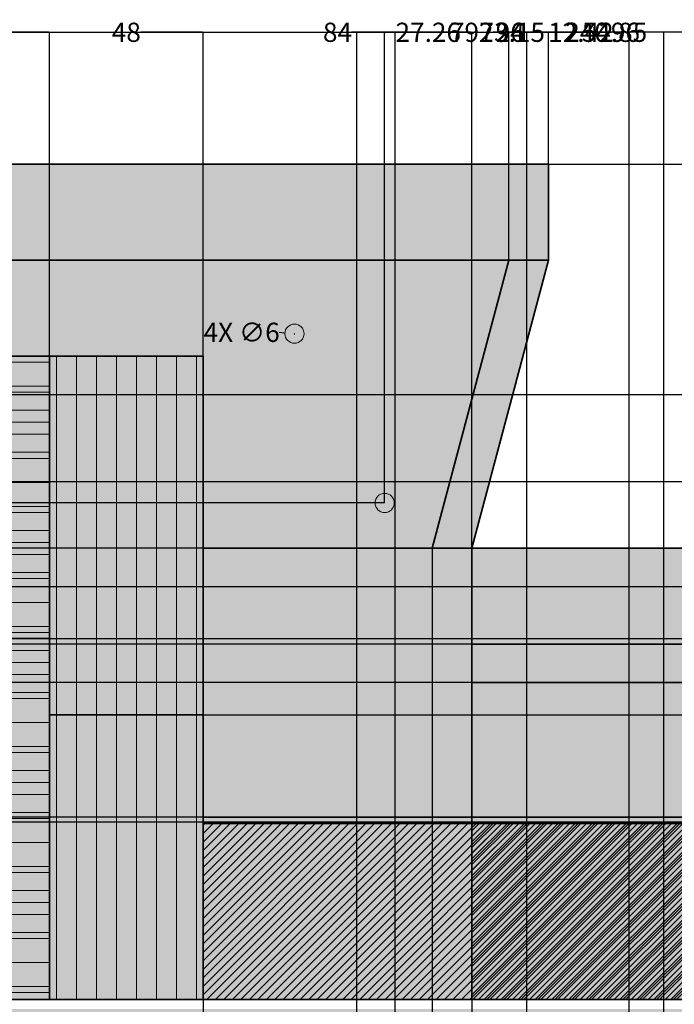
# Model space of a CAD drawing. Units: inches. Extents: x 148 to 1080, y 89 to 707.
# Tile 10 of 12: x 470 to 674, y 399 to 707. Entities that reach past the tile are written whole.
import ezdxf

# ---------------------------------------------------------------- set-up
doc = ezdxf.new("R2010")
doc.units = ezdxf.units.IN
doc.header["$MEASUREMENT"] = 0
for name, color, linetype, lineweight in [('A-ANNO-DIMS', 2, 'Continuous', 18), ('A-ELEV', 7, 'Continuous', 35), ('A-ELEV-PATT', 8, 'Continuous', 13), ('E-LITE', 3, 'Continuous', 18)]:
    doc.layers.add(name, color=color, linetype=linetype, lineweight=lineweight)
doc.styles.get("Standard").update_dxf_attribs({"font": 'arial.ttf'})
doc.dimstyles.get("Standard").update_dxf_attribs({"dimtxt": 6, "dimasz": 0.18, "dimexe": 0.18, "dimexo": 0.0625, "dimgap": 0.09, "dimtad": 0, "dimtih": 1, "dimtoh": 1, "dimdec": 0, "dimzin": 0, "dimdsep": 46, "dimlunit": 3, "dimtxsty": 'Standard', "dimcen": 0.09, "dimadec": 0, "dimazin": 0, "dimtfac": 1, "dimtdec": 0, "dimtofl": 0, "dimtmove": 0, "dimatfit": 3, "dimfxl": 1, "dimtolj": 1, "dimtzin": 0, "dimarcsym": 0})

# ---------------------------------------------------------------- blocks, each defined once
blk = doc.blocks.new('*D1')
at = {"layer": 'A-ANNO-DIMS', "color": 0, "lineweight": -2, "transparency": 16777216}
for p, q in [((215.02, 662.01), (215.02, 703.28)), ((215.2, 703.1), (604.32, 703.1)), ((1006.77, 703.1), (617.65, 703.1)), ((1006.95, 338.01), (1006.95, 703.28))]:
    blk.add_line(p, q, dxfattribs=at)
at = {"layer": 'A-ANNO-DIMS', "color": 0, "transparency": 16777216}
for points in [[(215.2, 703.13), (215.2, 703.07), (215.02, 703.1)], [(1006.77, 703.13), (1006.77, 703.07), (1006.95, 703.1)]]:
    blk.add_solid(points, dxfattribs=at)
at = {"layer": 'Defpoints', "color": 0, "transparency": 16777216}
for p in [(1006.95, 703.1), (215.02, 661.95), (1006.95, 337.95)]:
    blk.add_point(p, dxfattribs=at)
at = {"layer": 'A-ANNO-DIMS', "color": 0, "transparency": 16777216, "insert": (610.98, 703.1), "char_height": 6, "attachment_point": 5}
blk.add_mtext('\\A1;792', dxfattribs=at)
blk = doc.blocks.new('*D11')
at = {"layer": 'A-ANNO-DIMS', "color": 0, "lineweight": -2, "transparency": 16777216}
for p, q in [((395.02, 602.01), (395.02, 703.28)), ((395.2, 703.1), (432.64, 703.1)), ((478.84, 703.1), (441.4, 703.1)), ((479.02, 602.01), (479.02, 703.28))]:
    blk.add_line(p, q, dxfattribs=at)
at = {"layer": 'A-ANNO-DIMS', "color": 0, "transparency": 16777216}
for points in [[(395.2, 703.13), (395.2, 703.07), (395.02, 703.1)], [(478.84, 703.13), (478.84, 703.07), (479.02, 703.1)]]:
    blk.add_solid(points, dxfattribs=at)
at = {"layer": 'Defpoints', "color": 0, "transparency": 16777216}
for p in [(479.02, 703.1), (395.02, 601.95), (479.02, 601.95)]:
    blk.add_point(p, dxfattribs=at)
at = {"layer": 'A-ANNO-DIMS', "color": 0, "transparency": 16777216, "insert": (437.02, 703.1), "char_height": 6, "attachment_point": 5}
blk.add_mtext('\\A1;84', dxfattribs=at)
blk = doc.blocks.new('*D12')
at = {"layer": 'A-ANNO-DIMS', "color": 0, "lineweight": -2, "transparency": 16777216}
for p, q in [((479.02, 602.01), (479.02, 703.28)), ((479.2, 703.1), (498.51, 703.1)), ((526.84, 703.1), (507.53, 703.1)), ((527.02, 602.01), (527.02, 703.28))]:
    blk.add_line(p, q, dxfattribs=at)
at = {"layer": 'A-ANNO-DIMS', "color": 0, "transparency": 16777216}
for points in [[(479.2, 703.13), (479.2, 703.07), (479.02, 703.1)], [(526.84, 703.13), (526.84, 703.07), (527.02, 703.1)]]:
    blk.add_solid(points, dxfattribs=at)
at = {"layer": 'Defpoints', "color": 0, "transparency": 16777216}
for p in [(527.02, 703.1), (479.02, 601.95), (527.02, 601.95)]:
    blk.add_point(p, dxfattribs=at)
at = {"layer": 'A-ANNO-DIMS', "color": 0, "transparency": 16777216, "insert": (503.02, 703.1), "char_height": 6, "attachment_point": 5}
blk.add_mtext('\\A1;48', dxfattribs=at)
blk = doc.blocks.new('*D13')
at = {"layer": 'A-ANNO-DIMS', "color": 0, "lineweight": -2, "transparency": 16777216}
for p, q in [((527.02, 542.01), (527.02, 703.28)), ((527.2, 703.1), (564.64, 703.1)), ((610.84, 703.1), (573.4, 703.1)), ((611.02, 542.01), (611.02, 703.28))]:
    blk.add_line(p, q, dxfattribs=at)
at = {"layer": 'A-ANNO-DIMS', "color": 0, "transparency": 16777216}
for points in [[(527.2, 703.13), (527.2, 703.07), (527.02, 703.1)], [(610.84, 703.13), (610.84, 703.07), (611.02, 703.1)]]:
    blk.add_solid(points, dxfattribs=at)
at = {"layer": 'Defpoints', "color": 0, "transparency": 16777216}
for p in [(611.02, 703.1), (527.02, 541.95), (611.02, 541.95)]:
    blk.add_point(p, dxfattribs=at)
at = {"layer": 'A-ANNO-DIMS', "color": 0, "transparency": 16777216, "insert": (569.02, 703.1), "char_height": 6, "attachment_point": 5}
blk.add_mtext('\\A1;84', dxfattribs=at)
blk = doc.blocks.new('*D14')
at = {"layer": 'A-ANNO-DIMS', "color": 0, "lineweight": -2, "transparency": 16777216}
for p, q in [((611.02, 542.01), (611.02, 703.28)), ((611.2, 703.1), (654.63, 703.1)), ((706.84, 703.1), (663.41, 703.1)), ((707.02, 542.01), (707.02, 703.28))]:
    blk.add_line(p, q, dxfattribs=at)
at = {"layer": 'A-ANNO-DIMS', "color": 0, "transparency": 16777216}
for points in [[(611.2, 703.13), (611.2, 703.07), (611.02, 703.1)], [(706.84, 703.13), (706.84, 703.07), (707.02, 703.1)]]:
    blk.add_solid(points, dxfattribs=at)
at = {"layer": 'Defpoints', "color": 0, "transparency": 16777216}
for p in [(707.02, 703.1), (611.02, 541.95), (707.02, 541.95)]:
    blk.add_point(p, dxfattribs=at)
at = {"layer": 'A-ANNO-DIMS', "color": 0, "transparency": 16777216, "insert": (659.02, 703.1), "char_height": 6, "attachment_point": 5}
blk.add_mtext('\\A1;96', dxfattribs=at)
blk = doc.blocks.new('*D15')
at = {"layer": 'A-ANNO-DIMS', "color": 0, "lineweight": -2, "transparency": 16777216}
for p, q in [((611.02, 542.01), (611.02, 703.28)), ((611.2, 703.1), (618.59, 703.1)), ((634.84, 703.1), (627.45, 703.1)), ((635.02, 632.01), (635.02, 703.28))]:
    blk.add_line(p, q, dxfattribs=at)
at = {"layer": 'A-ANNO-DIMS', "color": 0, "transparency": 16777216}
for points in [[(611.2, 703.13), (611.2, 703.07), (611.02, 703.1)], [(634.84, 703.13), (634.84, 703.07), (635.02, 703.1)]]:
    blk.add_solid(points, dxfattribs=at)
at = {"layer": 'Defpoints', "color": 0, "transparency": 16777216}
for p in [(635.02, 703.1), (635.02, 631.95), (611.02, 541.95)]:
    blk.add_point(p, dxfattribs=at)
at = {"layer": 'A-ANNO-DIMS', "color": 0, "transparency": 16777216, "insert": (623.02, 703.1), "char_height": 6, "attachment_point": 5}
blk.add_mtext('\\A1;24', dxfattribs=at)
blk = doc.blocks.new('*D16')
at = {"layer": 'A-ANNO-DIMS', "color": 0, "lineweight": -2, "transparency": 16777216}
for p, q in [((527.02, 458.01), (527.02, 703.28)), ((527.2, 703.1), (640.26, 703.1)), ((766.84, 703.1), (653.78, 703.1)), ((767.02, 458.01), (767.02, 703.28))]:
    blk.add_line(p, q, dxfattribs=at)
at = {"layer": 'A-ANNO-DIMS', "color": 0, "transparency": 16777216}
for points in [[(527.2, 703.13), (527.2, 703.07), (527.02, 703.1)], [(766.84, 703.13), (766.84, 703.07), (767.02, 703.1)]]:
    blk.add_solid(points, dxfattribs=at)
at = {"layer": 'Defpoints', "color": 0, "transparency": 16777216}
for p in [(767.02, 703.1), (527.02, 457.95), (767.02, 457.95)]:
    blk.add_point(p, dxfattribs=at)
at = {"layer": 'A-ANNO-DIMS', "color": 0, "transparency": 16777216, "insert": (647.02, 703.1), "char_height": 6, "attachment_point": 5}
blk.add_mtext('\\A1;240', dxfattribs=at)
blk = doc.blocks.new('*D18')
at = {"layer": 'A-ANNO-DIMS', "color": 0, "lineweight": -2, "transparency": 16777216}
for p, q in [((635.08, 661.95), (1064.5, 661.95)), ((1064.32, 661.77), (1064.32, 401.1)), ((1064.32, 134.13), (1064.32, 394.79)), ((1007.01, 133.95), (1064.5, 133.95))]:
    blk.add_line(p, q, dxfattribs=at)
at = {"layer": 'A-ANNO-DIMS', "color": 0, "transparency": 16777216}
for points in [[(1064.29, 661.77), (1064.35, 661.77), (1064.32, 661.95)], [(1064.29, 134.13), (1064.35, 134.13), (1064.32, 133.95)]]:
    blk.add_solid(points, dxfattribs=at)
at = {"layer": 'Defpoints', "color": 0, "transparency": 16777216}
for p in [(635.02, 661.95), (1064.32, 661.95), (1006.95, 133.95)]:
    blk.add_point(p, dxfattribs=at)
at = {"layer": 'A-ANNO-DIMS', "color": 0, "transparency": 16777216, "insert": (1064.32, 397.95), "char_height": 6, "attachment_point": 5}
blk.add_mtext('\\A1;528', dxfattribs=at)
blk = doc.blocks.new('*D31')
at = {"layer": 'A-ANNO-DIMS', "color": 0, "lineweight": -2, "transparency": 16777216}
for p, q in [((587.06, 271.84), (587.06, 703.28)), ((587.24, 703.1), (613.42, 703.1)), ((660.03, 703.1), (633.85, 703.1)), ((660.21, 271.84), (660.21, 703.28))]:
    blk.add_line(p, q, dxfattribs=at)
at = {"layer": 'A-ANNO-DIMS', "color": 0, "transparency": 16777216}
for points in [[(587.24, 703.13), (587.24, 703.07), (587.06, 703.1)], [(660.03, 703.13), (660.03, 703.07), (660.21, 703.1)]]:
    blk.add_solid(points, dxfattribs=at)
at = {"layer": 'Defpoints', "color": 0, "transparency": 16777216}
for p in [(660.21, 703.1), (587.06, 271.77), (660.21, 271.77)]:
    blk.add_point(p, dxfattribs=at)
at = {"layer": 'A-ANNO-DIMS', "color": 0, "transparency": 16777216, "insert": (623.64, 703.1), "char_height": 6, "attachment_point": 5}
blk.add_mtext('\\A1;73.15', dxfattribs=at)
blk = doc.blocks.new('*D33')
at = {"layer": 'A-ANNO-DIMS', "color": 0, "lineweight": -2, "transparency": 16777216}
for p, q in [((575.02, 284.01), (575.02, 703.28)), ((575.2, 703.1), (618.63, 703.1)), ((670.84, 703.1), (627.41, 703.1)), ((671.02, 284.01), (671.02, 703.28))]:
    blk.add_line(p, q, dxfattribs=at)
at = {"layer": 'A-ANNO-DIMS', "color": 0, "transparency": 16777216}
for points in [[(575.2, 703.13), (575.2, 703.07), (575.02, 703.1)], [(670.84, 703.13), (670.84, 703.07), (671.02, 703.1)]]:
    blk.add_solid(points, dxfattribs=at)
at = {"layer": 'Defpoints', "color": 0, "transparency": 16777216}
for p in [(671.02, 703.1), (575.02, 283.95), (671.02, 283.95)]:
    blk.add_point(p, dxfattribs=at)
at = {"layer": 'A-ANNO-DIMS', "color": 0, "transparency": 16777216, "insert": (623.02, 703.1), "char_height": 6, "attachment_point": 5}
blk.add_mtext('\\A1;96', dxfattribs=at)
blk = doc.blocks.new('*D40')
at = {"layer": 'A-ANNO-DIMS', "color": 0, "lineweight": -2, "transparency": 16777216}
for p, q in [((526.96, 457.95), (160.42, 457.95)), ((160.6, 457.77), (160.6, 432.59)), ((160.6, 401.13), (160.6, 426.31)), ((526.96, 400.95), (160.42, 400.95))]:
    blk.add_line(p, q, dxfattribs=at)
at = {"layer": 'A-ANNO-DIMS', "color": 0, "transparency": 16777216}
for points in [[(160.57, 457.77), (160.63, 457.77), (160.6, 457.95)], [(160.57, 401.13), (160.63, 401.13), (160.6, 400.95)]]:
    blk.add_solid(points, dxfattribs=at)
at = {"layer": 'Defpoints', "color": 0, "transparency": 16777216}
for p in [(527.02, 457.95), (160.6, 400.95), (527.02, 400.95)]:
    blk.add_point(p, dxfattribs=at)
at = {"layer": 'A-ANNO-DIMS', "color": 0, "transparency": 16777216, "insert": (160.6, 429.45), "char_height": 6, "attachment_point": 5}
blk.add_mtext('\\A1;57', dxfattribs=at)
blk = doc.blocks.new('*D41')
at = {"layer": 'A-ANNO-DIMS', "color": 0, "lineweight": -2, "transparency": 16777216}
for p, q in [((610.96, 541.95), (160.42, 541.95)), ((160.6, 541.77), (160.6, 530.1)), ((160.6, 512.13), (160.6, 523.79)), ((610.96, 511.95), (160.42, 511.95))]:
    blk.add_line(p, q, dxfattribs=at)
at = {"layer": 'A-ANNO-DIMS', "color": 0, "transparency": 16777216}
for points in [[(160.57, 541.77), (160.63, 541.77), (160.6, 541.95)], [(160.57, 512.13), (160.63, 512.13), (160.6, 511.95)]]:
    blk.add_solid(points, dxfattribs=at)
at = {"layer": 'Defpoints', "color": 0, "transparency": 16777216}
for p in [(611.02, 541.95), (160.6, 511.95), (611.02, 511.95)]:
    blk.add_point(p, dxfattribs=at)
at = {"layer": 'A-ANNO-DIMS', "color": 0, "transparency": 16777216, "insert": (160.6, 526.95), "char_height": 6, "attachment_point": 5}
blk.add_mtext('\\A1;30', dxfattribs=at)
blk = doc.blocks.new('*D44')
at = {"layer": 'A-ANNO-DIMS', "color": 0, "lineweight": -2, "transparency": 16777216}
for p, q in [((550.8, 609.37), (552.41, 609.23)), ((555.58, 608.86), (555.58, 609.04)), ((555.49, 608.95), (555.67, 608.95))]:
    blk.add_line(p, q, dxfattribs=at)
at = {"layer": 'A-ANNO-DIMS', "color": 0, "transparency": 16777216}
blk.add_solid([(552.41, 609.26), (552.41, 609.2), (552.59, 609.21)], dxfattribs=at)
at = {"layer": 'Defpoints', "color": 0, "transparency": 16777216}
for p in [(552.59, 609.21), (558.57, 608.69)]:
    blk.add_point(p, dxfattribs=at)
at = {"layer": 'A-ANNO-DIMS', "color": 0, "transparency": 16777216, "insert": (539.07, 609.37), "char_height": 6, "attachment_point": 5}
blk.add_mtext('\\A1;4X ∅6', dxfattribs=at)
blk = doc.blocks.new('*D45')
at = {"layer": 'A-ANNO-DIMS', "color": 0, "lineweight": -2, "transparency": 16777216}
for p, q in [((583.76, 556.13), (583.76, 703.28)), ((583.94, 703.1), (587.13, 703.1)), ((610.84, 703.1), (607.65, 703.1)), ((611.02, 542.01), (611.02, 703.28))]:
    blk.add_line(p, q, dxfattribs=at)
at = {"layer": 'A-ANNO-DIMS', "color": 0, "transparency": 16777216}
for points in [[(583.94, 703.13), (583.94, 703.07), (583.76, 703.1)], [(610.84, 703.13), (610.84, 703.07), (611.02, 703.1)]]:
    blk.add_solid(points, dxfattribs=at)
at = {"layer": 'Defpoints', "color": 0, "transparency": 16777216}
for p in [(611.02, 703.1), (583.76, 556.07), (611.02, 541.95)]:
    blk.add_point(p, dxfattribs=at)
at = {"layer": 'A-ANNO-DIMS', "color": 0, "transparency": 16777216, "insert": (597.39, 703.1), "char_height": 6, "attachment_point": 5}
blk.add_mtext('\\A1;27.26', dxfattribs=at)
blk = doc.blocks.new('*D46')
at = {"layer": 'A-ANNO-DIMS', "color": 0, "lineweight": -2, "transparency": 16777216}
for p, q in [((583.7, 556.07), (160.42, 556.07)), ((160.6, 555.89), (160.6, 552.16)), ((160.6, 542.13), (160.6, 545.85)), ((598.54, 541.95), (160.42, 541.95))]:
    blk.add_line(p, q, dxfattribs=at)
at = {"layer": 'A-ANNO-DIMS', "color": 0, "transparency": 16777216}
for points in [[(160.57, 555.89), (160.63, 555.89), (160.6, 556.07)], [(160.57, 542.13), (160.63, 542.13), (160.6, 541.95)]]:
    blk.add_solid(points, dxfattribs=at)
at = {"layer": 'Defpoints', "color": 0, "transparency": 16777216}
for p in [(583.76, 556.07), (160.6, 541.95), (598.6, 541.95)]:
    blk.add_point(p, dxfattribs=at)
at = {"layer": 'A-ANNO-DIMS', "color": 0, "transparency": 16777216, "insert": (160.6, 549.01), "char_height": 6, "attachment_point": 5}
blk.add_mtext('\\A1;14.118', dxfattribs=at)
blk = doc.blocks.new('*D47')
at = {"layer": 'A-ANNO-DIMS', "color": 0, "lineweight": -2, "transparency": 16777216}
for p, q in [((628.17, 353.26), (628.17, 703.28)), ((628.35, 703.1), (645.36, 703.1)), ((682.84, 703.1), (665.83, 703.1)), ((683.02, 338.01), (683.02, 703.28))]:
    blk.add_line(p, q, dxfattribs=at)
at = {"layer": 'A-ANNO-DIMS', "color": 0, "transparency": 16777216}
for points in [[(628.35, 703.13), (628.35, 703.07), (628.17, 703.1)], [(682.84, 703.13), (682.84, 703.07), (683.02, 703.1)]]:
    blk.add_solid(points, dxfattribs=at)
at = {"layer": 'Defpoints', "color": 0, "transparency": 16777216}
for p in [(683.02, 703.1), (628.17, 353.2), (683.02, 337.95)]:
    blk.add_point(p, dxfattribs=at)
at = {"layer": 'A-ANNO-DIMS', "color": 0, "transparency": 16777216, "insert": (655.6, 703.1), "char_height": 6, "attachment_point": 5}
blk.add_mtext('\\A1;54.85', dxfattribs=at)
blk = doc.blocks.new('*D52')
at = {"layer": 'A-ANNO-DIMS', "color": 0, "lineweight": -2, "transparency": 16777216}
for p, q in [((610.96, 511.95), (160.42, 511.95)), ((160.6, 511.77), (160.6, 509.1)), ((160.6, 500.13), (160.6, 502.79)), ((610.96, 499.95), (160.42, 499.95))]:
    blk.add_line(p, q, dxfattribs=at)
at = {"layer": 'A-ANNO-DIMS', "color": 0, "transparency": 16777216}
for points in [[(160.57, 511.77), (160.63, 511.77), (160.6, 511.95)], [(160.57, 500.13), (160.63, 500.13), (160.6, 499.95)]]:
    blk.add_solid(points, dxfattribs=at)
at = {"layer": 'Defpoints', "color": 0, "transparency": 16777216}
for p in [(160.6, 511.95), (611.02, 511.95), (611.02, 499.95)]:
    blk.add_point(p, dxfattribs=at)
at = {"layer": 'A-ANNO-DIMS', "color": 0, "transparency": 16777216, "insert": (160.6, 505.95), "char_height": 6, "attachment_point": 5}
blk.add_mtext('\\A1;12.00', dxfattribs=at)
blk = doc.blocks.new('*D55')
at = {"layer": 'A-ANNO-DIMS', "color": 0, "lineweight": -2, "transparency": 16777216}
for p, q in [((598.6, 541.88), (598.6, 92.62)), ((611.02, 541.88), (611.02, 92.62)), ((598.78, 92.8), (610.84, 92.8)), ((611.02, 92.8), (611.2, 92.8))]:
    blk.add_line(p, q, dxfattribs=at)
at = {"layer": 'A-ANNO-DIMS', "color": 0, "transparency": 16777216}
for points in [[(598.78, 92.83), (598.78, 92.77), (598.6, 92.8)], [(610.84, 92.83), (610.84, 92.77), (611.02, 92.8)]]:
    blk.add_solid(points, dxfattribs=at)
at = {"layer": 'Defpoints', "color": 0, "transparency": 16777216}
for p in [(598.6, 541.95), (611.02, 541.95), (611.02, 92.8)]:
    blk.add_point(p, dxfattribs=at)
at = {"layer": 'A-ANNO-DIMS', "color": 0, "transparency": 16777216, "insert": (621.1, 92.8), "char_height": 6, "attachment_point": 5}
blk.add_mtext('\\A1;12.42', dxfattribs=at)
blk = doc.blocks.new('*D56')
at = {"layer": 'A-ANNO-DIMS', "color": 0, "lineweight": -2, "transparency": 16777216}
for p, q in [((622.6, 632.01), (622.6, 703.28)), ((622.78, 703.1), (634.84, 703.1)), ((635.02, 632.01), (635.02, 703.28)), ((635.02, 703.1), (635.2, 703.1))]:
    blk.add_line(p, q, dxfattribs=at)
at = {"layer": 'A-ANNO-DIMS', "color": 0, "transparency": 16777216}
for points in [[(622.78, 703.13), (622.78, 703.07), (622.6, 703.1)], [(634.84, 703.13), (634.84, 703.07), (635.02, 703.1)]]:
    blk.add_solid(points, dxfattribs=at)
at = {"layer": 'Defpoints', "color": 0, "transparency": 16777216}
for p in [(635.02, 703.1), (622.6, 631.95), (635.02, 631.95)]:
    blk.add_point(p, dxfattribs=at)
at = {"layer": 'A-ANNO-DIMS', "color": 0, "transparency": 16777216, "insert": (645.1, 703.1), "char_height": 6, "attachment_point": 5}
blk.add_mtext('\\A1;12.42', dxfattribs=at)
blk = doc.blocks.new('*D57')
at = {"layer": 'A-ANNO-DIMS', "color": 0, "lineweight": -2, "transparency": 16777216}
for p, q in [((527.02, 400.88), (527.02, 92.62)), ((611.02, 400.88), (611.02, 92.62)), ((527.2, 92.8), (558.81, 92.8)), ((610.84, 92.8), (579.23, 92.8))]:
    blk.add_line(p, q, dxfattribs=at)
at = {"layer": 'A-ANNO-DIMS', "color": 0, "transparency": 16777216}
for points in [[(527.2, 92.83), (527.2, 92.77), (527.02, 92.8)], [(610.84, 92.83), (610.84, 92.77), (611.02, 92.8)]]:
    blk.add_solid(points, dxfattribs=at)
at = {"layer": 'Defpoints', "color": 0, "transparency": 16777216}
for p in [(527.02, 400.95), (611.02, 400.95), (611.02, 92.8)]:
    blk.add_point(p, dxfattribs=at)
at = {"layer": 'A-ANNO-DIMS', "color": 0, "transparency": 16777216, "insert": (569.02, 92.8), "char_height": 6, "attachment_point": 5}
blk.add_mtext('\\A1;84.00', dxfattribs=at)
blk = doc.blocks.new('*D58')
at = {"layer": 'A-ANNO-DIMS', "color": 0, "lineweight": -2, "transparency": 16777216}
for p, q in [((611.02, 400.88), (611.02, 92.62)), ((695.02, 400.88), (695.02, 92.62)), ((611.2, 92.8), (642.81, 92.8)), ((694.84, 92.8), (663.23, 92.8))]:
    blk.add_line(p, q, dxfattribs=at)
at = {"layer": 'A-ANNO-DIMS', "color": 0, "transparency": 16777216}
for points in [[(611.2, 92.83), (611.2, 92.77), (611.02, 92.8)], [(694.84, 92.83), (694.84, 92.77), (695.02, 92.8)]]:
    blk.add_solid(points, dxfattribs=at)
at = {"layer": 'Defpoints', "color": 0, "transparency": 16777216}
for p in [(611.02, 400.95), (695.02, 400.95), (695.02, 92.8)]:
    blk.add_point(p, dxfattribs=at)
at = {"layer": 'A-ANNO-DIMS', "color": 0, "transparency": 16777216, "insert": (653.02, 92.8), "char_height": 6, "attachment_point": 5}
blk.add_mtext('\\A1;84.00', dxfattribs=at)
blk = doc.blocks.new('*D90')
at = {"layer": 'A-ANNO-DIMS', "color": 0, "lineweight": -2, "transparency": 16777216}
for p, q in [((527.08, 489.89), (1064.5, 489.89)), ((1064.32, 489.71), (1064.32, 448.57)), ((1064.32, 401.13), (1064.32, 442.27)), ((527.08, 400.95), (1064.5, 400.95))]:
    blk.add_line(p, q, dxfattribs=at)
at = {"layer": 'A-ANNO-DIMS', "color": 0, "transparency": 16777216}
for points in [[(1064.29, 489.71), (1064.35, 489.71), (1064.32, 489.89)], [(1064.29, 401.13), (1064.35, 401.13), (1064.32, 400.95)]]:
    blk.add_solid(points, dxfattribs=at)
at = {"layer": 'Defpoints', "color": 0, "transparency": 16777216}
for p in [(527.02, 489.89), (527.02, 400.95), (1064.32, 400.95)]:
    blk.add_point(p, dxfattribs=at)
at = {"layer": 'A-ANNO-DIMS', "color": 0, "transparency": 16777216, "insert": (1064.32, 445.42), "char_height": 6, "attachment_point": 5}
blk.add_mtext('\\A1;88.94', dxfattribs=at)
blk = doc.blocks.new('*D91')
at = {"layer": 'A-ANNO-DIMS', "color": 0, "lineweight": -2, "transparency": 16777216}
for p, q in [((479.08, 513.77), (1064.5, 513.77)), ((1064.32, 513.59), (1064.32, 460.51)), ((1064.32, 401.13), (1064.32, 454.21)), ((479.08, 400.95), (1064.5, 400.95))]:
    blk.add_line(p, q, dxfattribs=at)
at = {"layer": 'A-ANNO-DIMS', "color": 0, "transparency": 16777216}
for points in [[(1064.29, 513.59), (1064.35, 513.59), (1064.32, 513.77)], [(1064.29, 401.13), (1064.35, 401.13), (1064.32, 400.95)]]:
    blk.add_solid(points, dxfattribs=at)
at = {"layer": 'Defpoints', "color": 0, "transparency": 16777216}
for p in [(479.02, 513.77), (479.02, 400.95), (1064.32, 400.95)]:
    blk.add_point(p, dxfattribs=at)
at = {"layer": 'A-ANNO-DIMS', "color": 0, "transparency": 16777216, "insert": (1064.32, 457.36), "char_height": 6, "attachment_point": 5}
blk.add_mtext('\\A1;112.82', dxfattribs=at)
blk = doc.blocks.new('*D92')
at = {"layer": 'A-ANNO-DIMS', "color": 0, "lineweight": -2, "transparency": 16777216}
for p, q in [((389.08, 456.43), (1064.5, 456.43)), ((1064.32, 456.25), (1064.32, 431.84)), ((1064.32, 401.13), (1064.32, 425.53)), ((389.08, 400.95), (1064.5, 400.95))]:
    blk.add_line(p, q, dxfattribs=at)
at = {"layer": 'A-ANNO-DIMS', "color": 0, "transparency": 16777216}
for points in [[(1064.29, 456.25), (1064.35, 456.25), (1064.32, 456.43)], [(1064.29, 401.13), (1064.35, 401.13), (1064.32, 400.95)]]:
    blk.add_solid(points, dxfattribs=at)
at = {"layer": 'Defpoints', "color": 0, "transparency": 16777216}
for p in [(389.02, 456.43), (1064.32, 456.43), (389.02, 400.95)]:
    blk.add_point(p, dxfattribs=at)
at = {"layer": 'A-ANNO-DIMS', "color": 0, "transparency": 16777216, "insert": (1064.32, 428.69), "char_height": 6, "attachment_point": 5}
blk.add_mtext('\\A1;55.48', dxfattribs=at)
blk = doc.blocks.new('*D93')
at = {"layer": 'A-ANNO-DIMS', "color": 0, "lineweight": -2, "transparency": 16777216}
for p, q in [((389.08, 529.95), (1064.5, 529.95)), ((1064.32, 529.77), (1064.32, 496.34)), ((1064.32, 456.61), (1064.32, 490.03)), ((389.08, 456.43), (1064.5, 456.43))]:
    blk.add_line(p, q, dxfattribs=at)
at = {"layer": 'A-ANNO-DIMS', "color": 0, "transparency": 16777216}
for points in [[(1064.29, 529.77), (1064.35, 529.77), (1064.32, 529.95)], [(1064.29, 456.61), (1064.35, 456.61), (1064.32, 456.43)]]:
    blk.add_solid(points, dxfattribs=at)
at = {"layer": 'Defpoints', "color": 0, "transparency": 16777216}
for p in [(389.02, 529.95), (1064.32, 529.95), (389.02, 456.43)]:
    blk.add_point(p, dxfattribs=at)
at = {"layer": 'A-ANNO-DIMS', "color": 0, "transparency": 16777216, "insert": (1064.32, 493.19), "char_height": 6, "attachment_point": 5}
blk.add_mtext('\\A1;73.52', dxfattribs=at)
blk = doc.blocks.new('*D94')
at = {"layer": 'A-ANNO-DIMS', "color": 0, "lineweight": -2, "transparency": 16777216}
for p, q in [((389.08, 562.74), (1064.5, 562.74)), ((1064.32, 562.56), (1064.32, 549.5)), ((1064.32, 530.13), (1064.32, 543.19)), ((389.08, 529.95), (1064.5, 529.95))]:
    blk.add_line(p, q, dxfattribs=at)
at = {"layer": 'A-ANNO-DIMS', "color": 0, "transparency": 16777216}
for points in [[(1064.29, 562.56), (1064.35, 562.56), (1064.32, 562.74)], [(1064.29, 530.13), (1064.35, 530.13), (1064.32, 529.95)]]:
    blk.add_solid(points, dxfattribs=at)
at = {"layer": 'Defpoints', "color": 0, "transparency": 16777216}
for p in [(389.02, 562.74), (1064.32, 562.74), (389.02, 529.95)]:
    blk.add_point(p, dxfattribs=at)
at = {"layer": 'A-ANNO-DIMS', "color": 0, "transparency": 16777216, "insert": (1064.32, 546.34), "char_height": 6, "attachment_point": 5}
blk.add_mtext('\\A1;32.79', dxfattribs=at)
blk = doc.blocks.new('*D95')
at = {"layer": 'A-ANNO-DIMS', "color": 0, "lineweight": -2, "transparency": 16777216}
for p, q in [((389.08, 589.95), (1064.5, 589.95)), ((1064.32, 589.77), (1064.32, 579.44)), ((1064.32, 562.92), (1064.32, 573.24)), ((389.08, 562.74), (1064.5, 562.74))]:
    blk.add_line(p, q, dxfattribs=at)
at = {"layer": 'A-ANNO-DIMS', "color": 0, "transparency": 16777216}
for points in [[(1064.29, 589.77), (1064.35, 589.77), (1064.32, 589.95)], [(1064.29, 562.92), (1064.35, 562.92), (1064.32, 562.74)]]:
    blk.add_solid(points, dxfattribs=at)
at = {"layer": 'Defpoints', "color": 0, "transparency": 16777216}
for p in [(389.02, 589.95), (1064.32, 589.95), (389.02, 562.74)]:
    blk.add_point(p, dxfattribs=at)
at = {"layer": 'A-ANNO-DIMS', "color": 0, "transparency": 16777216, "insert": (1064.32, 576.34), "char_height": 6, "attachment_point": 5}
blk.add_mtext('\\A1;27.21', dxfattribs=at)

msp = doc.modelspace()

# ---------------------------------------------------------------- hatches: boundary and pattern name
at = {"layer": 'A-ELEV-PATT'}
h = msp.add_hatch(color=256, dxfattribs=at)
h.dxf.hatch_style = 1
h.paths.add_polyline_path([(635.0199, 661.9474), (611.0199, 661.9474), (215.0199, 661.9474), (215.0199, 631.9474), (611.0199, 631.9474), (635.0199, 631.9474)])
h.paths.add_polyline_path([(773.0199, 397.9474), (215.0199, 397.9474), (215.0199, 367.9474), (773.0199, 367.9474)])
h = msp.add_hatch(color=256, dxfattribs=at)
h.dxf.hatch_style = 1
h.paths.add_polyline_path([(622.6005, 631.9474), (611.0199, 631.9474), (215.0199, 631.9474), (251.0199, 542.9352), (251.0199, 601.9474), (527.0199, 601.9474), (527.0199, 541.9474), (598.6005, 541.9474)])
h.paths.add_polyline_path([(558.5775, 608.9493, -1), (552.5775, 608.9493, -1)], flags=16)
h.paths.add_polyline_path([(586.7589, 556.0652, -1), (580.7589, 556.0652, -1)], flags=16)
h.paths.add_polyline_path([(635.0199, 631.9474), (622.6005, 631.9474), (598.6005, 541.9474), (611.0199, 541.9474)])
h.paths.add_polyline_path([(773.0199, 367.9474), (215.0199, 367.9474), (251.0199, 337.9474), (251.0199, 349.9474), (527.0199, 349.9474), (527.0199, 337.9474), (734.0628, 337.9474)])
h.paths.add_polyline_path([(631.1736, 353.1958, -1), (625.1736, 353.1958, -1)], flags=16)
h.paths.add_polyline_path([(729.9419, 354.8591, -1), (723.9419, 354.8591, -1)], flags=16)
h = msp.add_hatch(color=256, dxfattribs=at)
h.dxf.hatch_style = 1
h.paths.add_polyline_path([(552.5775, 608.9493, 1), (558.5775, 608.9493, 1)])
h.paths.add_polyline_path([(586.7589, 556.0652, 1), (580.7589, 556.0652, 1)])
h.paths.add_polyline_path([(625.1736, 353.1958, 1), (631.1736, 353.1958, 1)])
h.paths.add_polyline_path([(723.9419, 354.8591, 1), (729.9419, 354.8591, 1)])
h = msp.add_hatch(color=256, dxfattribs=at)
h.dxf.hatch_style = 1
h.paths.add_polyline_path([(479.0199, 601.9474), (395.0199, 601.9474), (395.0199, 513.7706), (479.0199, 513.7706)])
h.paths.add_polyline_path([(527.0199, 489.89), (479.0199, 489.89), (479.0199, 400.9474), (527.0199, 400.9474)])
h = msp.add_hatch(dxfattribs=at)
h.set_pattern_fill('ANSI31', color=256, scale=60, angle=135)
h.paths.add_polyline_path([(479.0199, 601.9474), (395.0199, 601.9474), (395.0199, 513.7706), (479.0199, 513.7706)])
h.paths.add_polyline_path([(479.0199, 513.7706), (395.0199, 513.7706), (395.0199, 400.9474), (479.0199, 400.9474)])
h.paths.add_polyline_path([(683.0199, 337.9474), (527.0199, 337.9474), (527.0199, 283.9474), (683.0199, 283.9474)])
h = msp.add_hatch(dxfattribs=at)
h.set_pattern_fill('ANSI31', color=256, scale=75, angle=135)
h.paths.add_polyline_path([(479.0199, 601.9474), (395.0199, 601.9474), (395.0199, 513.7706), (479.0199, 513.7706)])
h.paths.add_polyline_path([(479.0199, 513.7706), (395.0199, 513.7706), (395.0199, 400.9474), (479.0199, 400.9474)])
h = msp.add_hatch(color=256, dxfattribs=at)
h.dxf.hatch_style = 1
h.paths.add_polyline_path([(527.0199, 601.9474), (479.0199, 601.9474), (479.0199, 489.89), (527.0199, 489.89)])
h = msp.add_hatch(dxfattribs=at)
h.set_pattern_fill('ANSI31', color=256, scale=50, angle=45)
h.paths.add_polyline_path([(527.0199, 601.9474), (479.0199, 601.9474), (479.0199, 489.89), (527.0199, 489.89)])
h.paths.add_polyline_path([(527.0199, 489.89), (479.0199, 489.89), (479.0199, 400.9474), (527.0199, 400.9474)])
h = msp.add_hatch(color=256, dxfattribs=at)
h.dxf.hatch_style = 1
h.paths.add_polyline_path([(707.0199, 511.9474), (707.0199, 541.9474), (611.0199, 541.9474), (611.0199, 511.9474)])
h.paths.add_polyline_path([(479.0199, 513.7706), (395.0199, 513.7706), (395.0199, 400.9474), (479.0199, 400.9474)])
h = msp.add_hatch(color=256, dxfattribs=at)
h.dxf.hatch_style = 1
h.paths.add_polyline_path([(611.0199, 541.9474), (527.0199, 541.9474), (527.0199, 511.9474), (611.0199, 511.9474)])
h = msp.add_hatch(color=256, dxfattribs=at)
h.dxf.hatch_style = 1
h.paths.add_polyline_path([(611.0199, 511.9474), (527.0199, 511.9474), (527.0199, 457.9474), (611.0199, 457.9474)])
h = msp.add_hatch(color=256, dxfattribs=at)
h.dxf.hatch_style = 1
h.paths.add_polyline_path([(694.7271, 511.9474), (611.0199, 511.9474), (611.0199, 499.9474), (692.0605, 499.9474)])
h.paths.add_polyline_path([(692.0605, 499.9474), (611.0199, 499.9474), (611.0199, 457.9474), (682.7271, 457.9474)])
h.paths.add_polyline_path([(704.3532, 499.9474), (692.0605, 499.9474), (682.7271, 457.9474), (695.0199, 457.9474)])
h.paths.add_polyline_path([(707.0199, 511.9474), (694.7271, 511.9474), (692.0605, 499.9474), (704.3532, 499.9474)])
h = msp.add_hatch(color=256, dxfattribs=at)
h.dxf.hatch_style = 1
h.paths.add_polyline_path([(695.0199, 457.9474), (611.0199, 457.9474), (611.0199, 455.9474), (695.0199, 455.9474)])
h.paths.add_polyline_path([(611.0199, 457.9474), (527.0199, 457.9474), (527.0199, 455.9474), (611.0199, 455.9474)])
h = msp.add_hatch(dxfattribs=at)
h.set_pattern_fill('ANSI31', color=256, scale=15)
h.paths.add_polyline_path([(611.0199, 455.9474), (527.0199, 455.9474), (527.0199, 400.9474), (611.0199, 400.9474)])
h.paths.add_polyline_path([(695.0199, 455.9474), (611.0199, 455.9474), (611.0199, 400.9474), (695.0199, 400.9474)])
h.paths.add_polyline_path([(765.0227, 455.9474), (695.0199, 455.9474), (695.0199, 400.9474), (710.0996, 400.9474)], flags=17)
h.paths.add_polyline_path([(767.0199, 455.117), (767.0199, 457.9474), (695.0199, 457.9474), (695.0199, 455.9474), (765.0227, 455.9474), (710.0996, 400.9474), (712.9261, 400.9474)])
h.paths.add_polyline_path([(767.0199, 455.117), (712.9261, 400.9474), (767.0199, 400.9474)])
h = msp.add_hatch(color=256, dxfattribs=at)
h.dxf.hatch_style = 1
h.paths.add_polyline_path([(611.0199, 455.9474), (527.0199, 455.9474), (527.0199, 400.9474), (611.0199, 400.9474)])
h.paths.add_polyline_path([(765.0227, 455.9474), (695.0199, 455.9474), (695.0199, 400.9474), (710.0996, 400.9474)])
h = msp.add_hatch(color=256, dxfattribs=at)
h.dxf.hatch_style = 1
h.paths.add_polyline_path([(695.0199, 455.9474), (611.0199, 455.9474), (611.0199, 400.9474), (695.0199, 400.9474)])
h.paths.add_polyline_path([(767.0199, 455.117), (712.9261, 400.9474), (767.0199, 400.9474)])
h = msp.add_hatch(dxfattribs=at)
h.set_pattern_fill('ANSI31', color=256, scale=10)
h.paths.add_polyline_path([(767.0199, 455.117), (712.9261, 400.9474), (767.0199, 400.9474)])
h.paths.add_polyline_path([(695.0199, 455.9474), (611.0199, 455.9474), (611.0199, 400.9474), (695.0199, 400.9474)])

# ---------------------------------------------------------------- linework, layer by layer
at = {"layer": 'A-ELEV'}
for p, q in [((215.0199, 661.9474), (611.0199, 661.9474)), ((611.0199, 661.9474), (635.0199, 661.9474)), ((635.0199, 631.9474), (635.0199, 661.9474)), ((215.0199, 631.9474), (611.0199, 631.9474)), ((622.6005, 631.9474), (598.6005, 541.9474)), ((635.0199, 631.9474), (611.0199, 541.9474)), ((611.0199, 631.9474), (635.0199, 631.9474)), ((251.0199, 601.9474), (527.0199, 601.9474)), ((479.0199, 400.9474), (479.0199, 601.9474)), ((527.0199, 400.9474), (527.0199, 601.9474)), ((527.0199, 541.9474), (707.0199, 541.9474)), ((611.0199, 400.9474), (611.0199, 541.9474)), ((479.0199, 513.7706), (395.0199, 513.7706)), ((611.0199, 511.9474), (707.0199, 511.9474)), ((611.0199, 499.9474), (704.3532, 499.9474)), ((527.0199, 489.89), (479.0199, 489.89)), ((527.0199, 457.9474), (767.0199, 457.9474)), ((527.0199, 455.9474), (765.0227, 455.9474)), ((215.0199, 400.9474), (773.0199, 400.9474))]:
    msp.add_line(p, q, dxfattribs=at)
at = {"layer": 'E-LITE'}
for centre in [(555.5775, 608.9493), (583.7589, 556.0652)]:
    msp.add_circle(centre, 3, dxfattribs=at)

# ---------------------------------------------------------------- dimensions: what is measured, and where the dimension line sits
at = {"layer": 'A-ANNO-DIMS'}
for base, p1, p2, override, picture, middle in [((1006.9492, 703.0974), (215.0199, 661.9474), (1006.9492, 337.9474), {"dimdec": 0, "dimlfac": 1, "dimrnd": 0, "dimzin": 0, "dimdsep": 46, "dimlunit": 2}, '*D1', (610.9845, 703.0974)), ((479.0199, 703.0974), (395.0199, 601.9474), (479.0199, 601.9474), {"dimdec": 0, "dimlfac": 1, "dimrnd": 0, "dimzin": 0, "dimdsep": 46, "dimlunit": 2}, '*D11', (437.0199, 703.0974)), ((527.0199, 703.0974), (479.0199, 601.9474), (527.0199, 601.9474), {"dimdec": 0, "dimlfac": 1, "dimrnd": 0, "dimzin": 0, "dimdsep": 46, "dimlunit": 2}, '*D12', (503.0199, 703.0974)), ((611.0199, 703.0974), (527.0199, 541.9474), (611.0199, 541.9474), {"dimdec": 0, "dimlfac": 1, "dimrnd": 0, "dimzin": 0, "dimdsep": 46, "dimlunit": 2}, '*D13', (569.0199, 703.0974)), ((767.0199, 703.0974), (527.0199, 457.9474), (767.0199, 457.9474), {"dimdec": 0, "dimlfac": 1, "dimrnd": 0, "dimzin": 0, "dimdsep": 46, "dimlunit": 2}, '*D16', (647.0199, 703.0974)), ((671.0199, 703.0974), (575.0199, 283.9474), (671.0199, 283.9474), {"dimdec": 0, "dimlfac": 1, "dimrnd": 0, "dimzin": 0, "dimdsep": 46, "dimlunit": 2}, '*D33', (623.0199, 703.0974)), ((611.0199, 703.0974), (583.7589, 556.0652), (611.0199, 541.9474), {"dimdec": 2, "dimlfac": 1, "dimrnd": 0, "dimzin": 0, "dimdsep": 46, "dimlunit": 2}, '*D45', (597.3894, 703.0974)), ((660.2092, 703.0974), (587.0631, 271.7747), (660.2092, 271.7747), {"dimdec": 2, "dimlfac": 1, "dimrnd": 0, "dimzin": 0, "dimdsep": 46, "dimlunit": 2}, '*D31', (623.6362, 703.0974)), ((707.0199, 703.0974), (611.0199, 541.9474), (707.0199, 541.9474), {"dimdec": 0, "dimlfac": 1, "dimrnd": 0, "dimzin": 0, "dimdsep": 46, "dimlunit": 2}, '*D14', (659.0199, 703.0974)), ((635.0199, 703.0974), (611.0199, 541.9474), (635.0199, 631.9474), {"dimdec": 0, "dimlfac": 1, "dimrnd": 0, "dimzin": 0, "dimdsep": 46, "dimlunit": 2}, '*D15', (623.0199, 703.0974)), ((635.0199, 703.0974), (622.6005, 631.9474), (635.0199, 631.9474), {"dimdec": 2, "dimlfac": 1, "dimrnd": 0, "dimzin": 0, "dimdsep": 46, "dimlunit": 2}, '*D56', (645.1002, 703.0974)), ((683.0199, 703.0974), (628.1736, 353.1958), (683.0199, 337.9474), {"dimdec": 2, "dimlfac": 1, "dimrnd": 0, "dimzin": 0, "dimdsep": 46, "dimlunit": 2}, '*D47', (655.5968, 703.0974)), ((611.0199, 92.7974), (598.6005, 541.9474), (611.0199, 541.9474), {"dimdec": 2, "dimlfac": 1, "dimrnd": 0, "dimzin": 0, "dimdsep": 46, "dimlunit": 2}, '*D55', (621.1002, 92.7974)), ((611.0199, 92.7974), (527.0199, 400.9474), (611.0199, 400.9474), {"dimdec": 2, "dimlfac": 1, "dimrnd": 0, "dimzin": 0, "dimdsep": 46, "dimlunit": 2}, '*D57', (569.0199, 92.7974)), ((695.0199, 92.7974), (611.0199, 400.9474), (695.0199, 400.9474), {"dimdec": 2, "dimlfac": 1, "dimrnd": 0, "dimzin": 0, "dimdsep": 46, "dimlunit": 2}, '*D58', (653.0199, 92.7974))]:
    dim = msp.add_linear_dim(base=base, p1=p1, p2=p2, dimstyle='Standard', override=override, dxfattribs=at)
    dim.commit()
    dim.dimension.update_dxf_attribs({"geometry": picture, "text_midpoint": middle})
for base, p1, p2, override, picture, middle in [((1064.325, 661.9474), (1006.9492, 133.9474), (635.0199, 661.9474), {"dimdec": 0, "dimlfac": 1, "dimrnd": 0, "dimzin": 0, "dimdsep": 46, "dimlunit": 2}, '*D18', (1064.325, 397.9474)), ((1064.325, 589.9474), (389.0199, 562.736), (389.0199, 589.9474), {"dimdec": 2, "dimlfac": 1, "dimrnd": 0, "dimzin": 0, "dimdsep": 46, "dimlunit": 2}, '*D95', (1064.325, 576.3417)), ((1064.325, 562.736), (389.0199, 529.9474), (389.0199, 562.736), {"dimdec": 2, "dimlfac": 1, "dimrnd": 0, "dimzin": 0, "dimdsep": 46, "dimlunit": 2}, '*D94', (1064.325, 546.3417)), ((160.5992, 541.9474), (583.7589, 556.0652), (598.6005, 541.9474), {"dimdec": 3, "dimlfac": 1, "dimrnd": 0, "dimzin": 0, "dimdsep": 46, "dimlunit": 2}, '*D46', (160.5992, 549.0063)), ((160.5992, 511.9474), (611.0199, 541.9474), (611.0199, 511.9474), {"dimdec": 0, "dimlfac": 1, "dimrnd": 0, "dimzin": 0, "dimdsep": 46, "dimlunit": 2}, '*D41', (160.5992, 526.9474)), ((1064.325, 529.9474), (389.0199, 456.4274), (389.0199, 529.9474), {"dimdec": 2, "dimlfac": 1, "dimrnd": 0, "dimzin": 0, "dimdsep": 46, "dimlunit": 2}, '*D93', (1064.325, 493.1874)), ((1064.325, 400.9474), (479.0199, 513.7706), (479.0199, 400.9474), {"dimdec": 2, "dimlfac": 1, "dimrnd": 0, "dimzin": 0, "dimdsep": 46, "dimlunit": 2}, '*D91', (1064.325, 457.359)), ((160.5992, 511.9474), (611.0199, 499.9474), (611.0199, 511.9474), {"dimdec": 2, "dimlfac": 1, "dimrnd": 0, "dimzin": 0, "dimdsep": 46, "dimlunit": 2}, '*D52', (160.5992, 505.9474)), ((1064.325, 400.9474), (527.0199, 489.89), (527.0199, 400.9474), {"dimdec": 2, "dimlfac": 1, "dimrnd": 0, "dimzin": 0, "dimdsep": 46, "dimlunit": 2}, '*D90', (1064.325, 445.4187)), ((160.5992, 400.9474), (527.0199, 457.9474), (527.0199, 400.9474), {"dimdec": 0, "dimlfac": 1, "dimrnd": 0, "dimzin": 0, "dimdsep": 46, "dimlunit": 2}, '*D40', (160.5992, 429.4474)), ((1064.325, 456.4274), (389.0199, 400.9474), (389.0199, 456.4274), {"dimdec": 2, "dimlfac": 1, "dimrnd": 0, "dimzin": 0, "dimdsep": 46, "dimlunit": 2}, '*D92', (1064.325, 428.6874))]:
    dim = msp.add_linear_dim(base=base, p1=p1, p2=p2, angle=90, dimstyle='Standard', override=override, dxfattribs=at)
    dim.commit()
    dim.dimension.update_dxf_attribs({"geometry": picture, "text_midpoint": middle})
dim = msp.add_diameter_dim_2p(p1=(558.566, 608.6871), p2=(552.589, 609.2116), text='4X <>', dimstyle='Standard', override={"dimdec": 0, "dimlfac": 1, "dimrnd": 0, "dimzin": 0, "dimdsep": 46, "dimlunit": 2}, dxfattribs=at)
dim.commit()
dim.dimension.update_dxf_attribs({"geometry": '*D44', "text_midpoint": (550.7959, 609.3689), "dimtype": 163})

doc.saveas('drawing.dxf')
